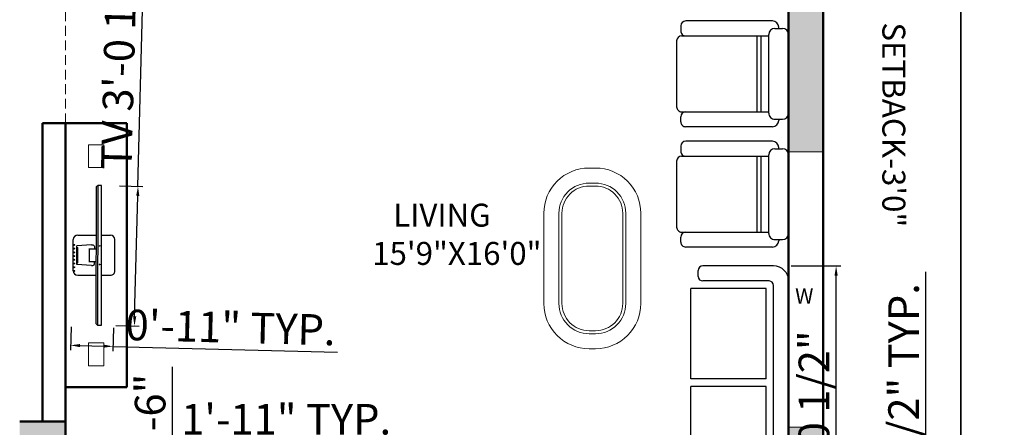
# Model space of a CAD drawing. Units: inches. Extents: x 3354 to 4308, y 1668 to 2317.
# Tile 5 of 11: x 3534 to 3792, y 1960 to 2066. Entities that reach past the tile are written whole.
import ezdxf

# ---------------------------------------------------------------- set-up
doc = ezdxf.new("R2010")
doc.units = ezdxf.units.IN
doc.linetypes.add('DASHED', pattern=[19.05, 12.7, -6.35])
for name, color, linetype, lineweight in [('A-ANNO-DIMS', 2, 'Continuous', 18), ('A-ANNO-TEXT', 7, 'Continuous', 18), ('A-AREA-IDEN', 3, 'Continuous', 18), ('A-FLOR-OVHD', 8, 'DASHED', 18), ('A-FURN', 8, 'Continuous', 18), ('A-GLAZ', 4, 'Continuous', 18), ('A-WALL', 7, 'Continuous', 50), ('A-WALL-PATT', 8, 'Continuous', 13), ('C-PROP', 1, 'Continuous', 35)]:
    doc.layers.add(name, color=color, linetype=linetype, lineweight=lineweight)
for name, color, linetype in [('M40-KOLTUKSUNGERI', 136, 'Continuous'), ('window', 130, 'Continuous'), ('wood', 26, 'Continuous')]:
    doc.layers.add(name, color=color, linetype=linetype)
doc.styles.get("Standard").update_dxf_attribs({"font": 'arial.ttf'})
doc.dimstyles.new('ISO-25', dxfattribs={"dimtxt": 8, "dimasz": 2.5, "dimexe": 1.25, "dimexo": 0.625, "dimtad": 1, "dimdec": 1, "dimlunit": 3, "dimtxsty": 'Standard', "dimcen": 2.5, "dimadec": 0, "dimazin": 0, "dimtfac": 1, "dimtdec": 1, "dimtmove": 0, "dimatfit": 3, "dimfxl": 1, "dimarcsym": 0})

# ---------------------------------------------------------------- blocks, each defined once
blk = doc.blocks.new('TV')
at = {"color": 0}
for p, q in [((3967.27, 1784.85), (3967.05, 1784.65)), ((3967.76, 1763.68), (3967.54, 1763.86))]:
    blk.add_line(p, q, dxfattribs=at)
at = {"layer": 'window'}
for p, q in [((3967.54, 1763.86), (3967.05, 1784.65)), ((3964.41, 1777.23), (3967.22, 1777.3)), ((3968.01, 1777.32), (3969.36, 1777.35)), ((3966.53, 1775.82), (3964.33, 1775.61)), ((3964.34, 1775.34), (3964.45, 1775.34)), ((3964.34, 1775.31), (3964.43, 1775.32)), ((3966.14, 1775.2), (3967.01, 1775.22)), ((3966.14, 1775.18), (3967.27, 1775.2)), ((3966.14, 1775.18), (3966.14, 1775.2)), ((3966.3, 1773.29), (3966.26, 1775.18)), ((3964.39, 1773.06), (3964.48, 1773.06)), ((3964.39, 1773.04), (3964.5, 1773.04)), ((3966.19, 1773.28), (3967.31, 1773.31)), ((3966.19, 1773.26), (3967.05, 1773.28)), ((3966.19, 1773.26), (3966.19, 1773.28)), ((3966.61, 1772.66), (3964.4, 1772.77)), ((3964.55, 1771.15), (3967.36, 1771.22)), ((3968.15, 1771.24), (3969.5, 1771.27))]:
    blk.add_line(p, q, dxfattribs=at)
for points in [[(3968.33, 1763.69), (3967.83, 1784.86), (3967.27, 1784.85), (3967.76, 1763.68), (3968.33, 1763.69)], [(3963.86, 1771.81), (3963.75, 1776.54)], [(3970.16, 1771.96), (3970.05, 1776.69)], [(3964.4, 1772.77), (3964.33, 1775.61)], [(3964.48, 1773.06), (3964.43, 1775.32)], [(3964.5, 1773.04), (3964.45, 1775.34)]]:
    blk.add_lwpolyline(points, dxfattribs=at)
for points in [[(3966.53, 1775.82, -0.263666), (3966.93, 1775.69), (3967, 1775.57), (3967.01, 1775.22)], [(3966.61, 1772.66, 0.263666), (3967, 1772.81), (3967.06, 1772.93), (3967.05, 1773.28)]]:
    blk.add_lwpolyline(points, format="xyb", dxfattribs=at)
for centre, radius in [((3963.91, 1775.73), 0.0679), ((3963.93, 1775.17), 0.0679), ((3963.94, 1774.6), 0.0679), ((3967.77, 1775.68), 0.0451), ((3963.95, 1774.04), 0.0679), ((3963.97, 1773.48), 0.0679), ((3963.98, 1772.92), 0.0679), ((3963.99, 1772.35), 0.0679), ((3964.01, 1771.79), 0.0679), ((3967.83, 1772.86), 0.0451)]:
    blk.add_circle(centre, radius, dxfattribs=at)
for centre, start, end in [((3964.42, 1776.56), 91.3414, 181.3414), ((3969.38, 1776.67), 1.3414, 91.3414), ((3964.53, 1771.83), 181.3414, 271.3414), ((3969.49, 1771.94), 271.3414, 1.3414)]:
    blk.add_arc(centre, 0.676, start, end, dxfattribs=at)
blk = doc.blocks.new('sofa 1')
at = {"layer": 'M40-KOLTUKSUNGERI'}
for p, q in [((72.87, 57.09), (54.36, 57.09)), ((53.18, 54.33), (53.18, 55.91)), ((71.69, 53.15), (54.36, 53.15)), ((72.87, -20.47), (72.87, 51.97)), ((76.8, -21.65), (76.8, 53.15)), ((51.21, 27.56), (51.21, 51.18)), ((70.9, 51.18), (51.21, 51.18)), ((70.9, 27.56), (70.9, 51.18)), ((70.9, 27.56), (51.21, 27.56)), ((51.21, 1.97), (51.21, 25.59)), ((70.9, 25.59), (51.21, 25.59)), ((70.9, 1.97), (70.9, 25.59)), ((0, -19.69), (0, 0)), ((0, -19.69), (0, 0)), ((23.62, 0), (0, 0)), ((23.62, -19.69), (23.62, 0)), ((25.59, -19.69), (25.59, 0)), ((49.21, 0), (25.59, 0)), ((49.21, -19.69), (49.21, 0)), ((70.9, 1.97), (51.21, 1.97)), ((70.9, 0), (51.21, 0)), ((51.21, -19.69), (51.21, 0)), ((70.9, -19.69), (70.9, 0)), ((-3.15, -1.97), (-4.72, -1.97)), ((-5.91, -21.65), (-5.91, -3.15)), ((-1.97, -20.47), (-1.97, -3.15)), ((23.62, -19.69), (0, -19.69)), ((49.21, -19.69), (25.59, -19.69)), ((70.9, -19.69), (51.21, -19.69)), ((71.69, -21.65), (-0.79, -21.65)), ((72.87, -25.59), (-1.97, -25.59))]:
    blk.add_line(p, q, dxfattribs=at)
for centre, radius, start, end in [((54.36, 55.91), 1.18, 90, 180), ((72.87, 53.15), 3.94, 0, 90), ((54.36, 54.33), 1.18, 180, 270), ((71.69, 51.97), 1.18, 0, 90), ((-4.72, -3.15), 1.18, 90, 180), ((-3.15, -3.15), 1.18, 0, 90), ((-0.79, -20.47), 1.18, 180, 270), ((71.69, -20.47), 1.18, 270, 0), ((-1.97, -21.65), 3.94, 180, 270), ((72.87, -21.65), 3.94, 270, 0)]:
    blk.add_arc(centre, radius, start, end, dxfattribs=at)
blk = doc.blocks.new('A$C38B70996')
at = {"layer": 'wood'}
for p, q in [((0.11, 0.9), (0.74, 0.9)), ((0.06, 0.82), (0.05, 0.82)), ((0.06, 0.79), (0.06, 0.85)), ((0.79, 0.79), (0.79, 0.85)), ((0.79, 0.82), (0.8, 0.82)), ((0, 0.77), (0, 0.073)), ((0.74, 0.74), (0.11, 0.74)), ((0.12, 0.04), (0.12, 0.74)), ((0.73, 0.04), (0.73, 0.74)), ((0.85, 0.77), (0.85, 0.073)), ((0.73, 0.68), (0.12, 0.68)), ((0.73, 0.647), (0.12, 0.647)), ((0.04, 0.033), (0.08, 0.033)), ((0.16, 0), (0.69, 0)), ((0.81, 0.033), (0.77, 0.033))]:
    blk.add_line(p, q, dxfattribs=at)
for centre, radius, start, end in [((0.11, 0.85), 0.05, 90, 180), ((0.74, 0.85), 0.05, 0, 90), ((0.05, 0.77), 0.05, 90, 180), ((0.8, 0.77), 0.05, 360, 90), ((0.11, 0.79), 0.05, 180, 270), ((0.74, 0.79), 0.05, 270, 0), ((0.04, 0.073), 0.04, 180, 270), ((0.08, 0.073), 0.04, 270, 0), ((0.16, 0.04), 0.04, 180, 270), ((0.69, 0.04), 0.04, 270, 360), ((0.77, 0.073), 0.04, 180, 270), ((0.81, 0.073), 0.04, 270, 360)]:
    blk.add_arc(centre, radius, start, end, dxfattribs=at)
blk = doc.blocks.new('*D53')
at = {"layer": 'A-ANNO-DIMS', "color": 0, "lineweight": -2, "transparency": 16777216}
for p, q in [((3550.48, 1952.98), (3550.48, 1957.48)), ((3552.98, 1956.23), (3571.19, 1956.23)), ((3573.69, 1952.98), (3573.69, 1957.48)), ((3573.69, 1956.23), (3631.67, 1956.23))]:
    blk.add_line(p, q, dxfattribs=at)
at = {"layer": 'A-ANNO-DIMS', "color": 0, "transparency": 16777216}
for points in [[(3552.98, 1956.64), (3552.98, 1955.81), (3550.48, 1956.23)], [(3571.19, 1956.64), (3571.19, 1955.81), (3573.69, 1956.23)]]:
    blk.add_solid(points, dxfattribs=at)
at = {"layer": 'Defpoints', "color": 0, "transparency": 16777216}
for p in [(3573.69, 1956.23), (3550.48, 1952.36), (3573.69, 1952.36)]:
    blk.add_point(p, dxfattribs=at)
at = {"layer": 'A-ANNO-DIMS', "color": 0, "transparency": 16777216, "insert": (3603.93, 1960.87), "char_height": 8, "attachment_point": 5}
blk.add_mtext('1\'-11" TYP.', dxfattribs=at)
blk = doc.blocks.new('*D66')
at = {"layer": 'A-ANNO-DIMS', "color": 0, "lineweight": -2, "transparency": 16777216}
for p, q in [((3565.2, 2022.8), (3567.45, 2111.51)), ((3560.34, 2022.92), (3566.45, 2022.77)), ((3564.33, 1988.78), (3565.13, 2020.3)), ((3559.42, 1986.4), (3565.52, 1986.25))]:
    blk.add_line(p, q, dxfattribs=at)
at = {"layer": 'A-ANNO-DIMS', "color": 0, "transparency": 16777216}
for points in [[(3564.72, 2020.31), (3565.55, 2020.29), (3565.2, 2022.8)], [(3563.92, 1988.79), (3564.75, 1988.77), (3564.27, 1986.28)]]:
    blk.add_solid(points, dxfattribs=at)
at = {"layer": 'Defpoints', "color": 0, "transparency": 16777216}
for p in [(3559.72, 2022.94), (3565.2, 2022.8), (3558.79, 1986.42)]:
    blk.add_point(p, dxfattribs=at)
at = {"layer": 'A-ANNO-DIMS', "color": 0, "transparency": 16777216, "insert": (3561.6, 2068.53), "char_height": 8, "attachment_point": 5, "rotation": 88.5431}
blk.add_mtext('TV 3\'-0 1/2" TYP.', dxfattribs=at)
blk = doc.blocks.new('*D67')
at = {"layer": 'A-ANNO-DIMS', "color": 0, "lineweight": -2, "transparency": 16777216}
for p, q in [((3547.7, 1986.08), (3547.54, 1979.97)), ((3558.78, 1985.79), (3558.62, 1979.69)), ((3550.07, 1981.16), (3556.15, 1981)), ((3558.65, 1980.94), (3617.36, 1979.45))]:
    blk.add_line(p, q, dxfattribs=at)
at = {"layer": 'A-ANNO-DIMS', "color": 0, "transparency": 16777216}
for points in [[(3550.08, 1981.57), (3550.06, 1980.74), (3547.57, 1981.22)], [(3556.16, 1981.42), (3556.14, 1980.59), (3558.65, 1980.94)]]:
    blk.add_solid(points, dxfattribs=at)
at = {"layer": 'Defpoints', "color": 0, "transparency": 16777216}
for p in [(3547.71, 1986.7), (3558.79, 1986.42), (3558.65, 1980.94)]:
    blk.add_point(p, dxfattribs=at)
at = {"layer": 'A-ANNO-DIMS', "color": 0, "transparency": 16777216, "insert": (3589.38, 1984.87), "char_height": 8, "attachment_point": 5, "rotation": 358.5431}
blk.add_mtext('0\'-11" TYP.', dxfattribs=at)
blk = doc.blocks.new('*D70')
at = {"layer": 'A-ANNO-DIMS', "color": 0, "lineweight": -2, "transparency": 16777216}
for p, q in [((3771.12, 1859.52), (3771.12, 2000.47)), ((3761.34, 1859.52), (3772.37, 1859.52)), ((3771.12, 1792.61), (3771.12, 1857.02)), ((3761.34, 1790.11), (3772.37, 1790.11))]:
    blk.add_line(p, q, dxfattribs=at)
at = {"layer": 'A-ANNO-DIMS', "color": 0, "transparency": 16777216}
for points in [[(3770.71, 1857.02), (3771.54, 1857.02), (3771.12, 1859.52)], [(3770.71, 1792.61), (3771.54, 1792.61), (3771.12, 1790.11)]]:
    blk.add_solid(points, dxfattribs=at)
at = {"layer": 'Defpoints', "color": 0, "transparency": 16777216}
for p in [(3760.71, 1859.52), (3771.12, 1859.52), (3760.71, 1790.11)]:
    blk.add_point(p, dxfattribs=at)
at = {"layer": 'A-ANNO-DIMS', "color": 0, "transparency": 16777216, "insert": (3766.36, 1931.24), "char_height": 8, "attachment_point": 5, "rotation": 90}
blk.add_mtext('MOTORBIKE 5\'-9 1/2" TYP.', dxfattribs=at)
blk = doc.blocks.new('*D74')
at = {"layer": 'A-ANNO-DIMS', "color": 0, "lineweight": -2, "transparency": 16777216}
for p, q in [((3574.18, 1883.3), (3574.18, 1975.62)), ((3581.65, 1883.3), (3572.93, 1883.3)), ((3574.18, 1831.8), (3574.18, 1880.8)), ((3581.65, 1829.3), (3572.93, 1829.3))]:
    blk.add_line(p, q, dxfattribs=at)
at = {"layer": 'A-ANNO-DIMS', "color": 0, "transparency": 16777216}
for points in [[(3573.76, 1880.8), (3574.59, 1880.8), (3574.18, 1883.3)], [(3573.76, 1831.8), (3574.59, 1831.8), (3574.18, 1829.3)]]:
    blk.add_solid(points, dxfattribs=at)
at = {"layer": 'Defpoints', "color": 0, "transparency": 16777216}
for p in [(3574.18, 1883.3), (3582.28, 1883.3), (3582.28, 1829.3)]:
    blk.add_point(p, dxfattribs=at)
at = {"layer": 'A-ANNO-DIMS', "color": 0, "transparency": 16777216, "insert": (3569.41, 1930.71), "char_height": 8, "attachment_point": 5, "rotation": 90}
blk.add_mtext('MAIN DOOR 4\'-6"', dxfattribs=at)
blk = doc.blocks.new('*D87')
at = {"layer": 'A-ANNO-DIMS', "color": 0, "lineweight": -2, "transparency": 16777216}
for p, q in [((3735.9, 2001.97), (3748.93, 2001.97)), ((3747.68, 1921.8), (3747.68, 1999.47)), ((3735.9, 1919.3), (3748.93, 1919.3))]:
    blk.add_line(p, q, dxfattribs=at)
at = {"layer": 'A-ANNO-DIMS', "color": 0, "transparency": 16777216}
for points in [[(3747.27, 1999.47), (3748.1, 1999.47), (3747.68, 2001.97)], [(3747.27, 1921.8), (3748.1, 1921.8), (3747.68, 1919.3)]]:
    blk.add_solid(points, dxfattribs=at)
at = {"layer": 'Defpoints', "color": 0, "transparency": 16777216}
for p in [(3735.28, 2001.97), (3747.68, 2001.97), (3735.28, 1919.3)]:
    blk.add_point(p, dxfattribs=at)
at = {"layer": 'A-ANNO-DIMS', "color": 0, "transparency": 16777216, "insert": (3742.92, 1960.64), "char_height": 8, "attachment_point": 5, "rotation": 90}
blk.add_mtext('6\'-10 1/2"', dxfattribs=at)
blk = doc.blocks.new('*D88')
at = {"layer": 'A-ANNO-DIMS', "color": 0, "lineweight": -2, "transparency": 16777216}
for p, q in [((3405.28, 2080.67), (3405.28, 2074.65)), ((3441.28, 2080.67), (3441.28, 2074.65)), ((3407.78, 2075.9), (3438.78, 2075.9)), ((3441.28, 2075.9), (3543.5, 2075.9))]:
    blk.add_line(p, q, dxfattribs=at)
at = {"layer": 'A-ANNO-DIMS', "color": 0, "transparency": 16777216}
for points in [[(3407.78, 2076.31), (3407.78, 2075.48), (3405.28, 2075.9)], [(3438.78, 2076.31), (3438.78, 2075.48), (3441.28, 2075.9)]]:
    blk.add_solid(points, dxfattribs=at)
at = {"layer": 'Defpoints', "color": 0, "transparency": 16777216}
for p in [(3405.28, 2081.3), (3441.28, 2081.3), (3441.28, 2075.9)]:
    blk.add_point(p, dxfattribs=at)
at = {"layer": 'A-ANNO-DIMS', "color": 0, "transparency": 16777216, "insert": (3493.64, 2080.66), "char_height": 8, "attachment_point": 5}
blk.add_mtext('RANGE OVEN 3\'-0"', dxfattribs=at)

msp = doc.modelspace()

# ---------------------------------------------------------------- hatches: boundary and pattern name
at = {"layer": 'A-WALL-PATT', "transparency": 33554687}
h = msp.add_hatch(color=256, dxfattribs=at)
h.dxf.hatch_style = 1
h.paths.add_polyline_path([(3546.28, 1829.3), (3552.28, 1829.3), (3552.28, 1838.3), (3546.28, 1838.3), (3546.28, 1910.3), (3582.28, 1910.3), (3582.28, 1919.3), (3546.28, 1919.3), (3546.28, 1961.3), (3534.28, 1961.3), (3534.28, 1955.3), (3537.28, 1955.3), (3537.28, 1808.3), (3516.28, 1808.3), (3516.28, 1799.3), (3546.28, 1799.3)])
h.paths.add_polyline_path([(3672.28, 1919.3), (3656.51, 1919.3), (3630.28, 1919.3), (3630.28, 1910.3), (3642.28, 1910.3), (3642.28, 1838.3), (3630.28, 1838.3), (3630.28, 1835.3), (3630.28, 1829.3), (3642.28, 1829.3), (3642.28, 1799.3), (3651.28, 1799.3), (3651.28, 1910.3), (3672.28, 1910.3)])
h.paths.add_polyline_path([(3744.28, 1959.8), (3735.28, 1959.8), (3735.28, 1923.23), (3735.28, 1919.3), (3714.28, 1919.3), (3714.28, 1910.3), (3744.28, 1910.3)])
h.paths.add_polyline_path([(3744.28, 2072.3), (3735.28, 2072.3), (3735.28, 2031.8), (3744.28, 2031.8)])
h.paths.add_polyline_path([(3744.28, 2150.3), (3735.28, 2150.3), (3735.28, 2108.3), (3744.28, 2108.3)])
h.paths.add_polyline_path([(3744.28, 2258.3), (3705.28, 2258.3), (3705.28, 2249.3), (3735.28, 2249.3), (3735.28, 2210.3), (3744.28, 2210.3)])
h.paths.add_polyline_path([(3633.28, 2258.3), (3583.78, 2258.3), (3583.78, 2249.3), (3588.24, 2249.3), (3597.28, 2249.3), (3597.28, 2165.3), (3594.28, 2165.3), (3594.28, 2159.3), (3597.28, 2159.3), (3597.28, 2117.3), (3594.28, 2117.3), (3594.28, 2111.3), (3603.28, 2111.3), (3603.28, 2249.3), (3633.28, 2249.3)])
h.paths.add_polyline_path([(3559.78, 2258.3), (3492.28, 2258.3), (3492.28, 2249.3), (3537.28, 2249.3), (3537.28, 2117.3), (3534.28, 2117.3), (3534.28, 2111.3), (3564.28, 2111.3), (3564.28, 2117.3), (3546.28, 2117.3), (3546.28, 2159.3), (3564.28, 2159.3), (3564.28, 2165.3), (3546.28, 2165.3), (3546.28, 2249.3), (3559.78, 2249.3)])
h.paths.add_polyline_path([(3450.28, 2258.3), (3396.28, 2258.3), (3396.28, 1799.3), (3474.28, 1799.3), (3474.28, 1808.3), (3405.28, 1808.3), (3405.28, 1955.3), (3498.28, 1955.3), (3498.28, 1961.3), (3405.28, 1961.3), (3405.28, 2111.3), (3498.28, 2111.3), (3498.28, 2117.3), (3405.28, 2117.3), (3405.28, 2249.3), (3450.28, 2249.3)])
h.paths.add_polyline_path([(3582.28, 1838.3), (3576.28, 1838.3), (3576.28, 1829.3), (3582.28, 1829.3)], flags=17)

# ---------------------------------------------------------------- linework, layer by layer
at = {"layer": 'A-FLOR-OVHD', "ltscale": 0.2}
msp.add_line((3546.28, 2039.3), (3546.28, 2111.3), dxfattribs=at)
at = {"layer": 'A-FURN'}
for points in [[(3556.28, 2027.67), (3552.28, 2027.67), (3552.28, 2033.67), (3556.28, 2033.67)], [(3556.28, 1981.88), (3552.28, 1981.88), (3552.28, 1975.88), (3556.28, 1975.88)]]:
    msp.add_lwpolyline(points, close=True, dxfattribs=at)
for points in [[(3696.63, 2015.76), (3696.63, 1992.14, -0.414214), (3684.82, 1980.33), (3683.1, 1980.33, -0.414214), (3671.29, 1992.14), (3671.29, 2015.76, -0.414214), (3683.1, 2027.57), (3684.82, 2027.57, -0.414214)], [(3692.7, 2015.76), (3692.7, 1992.14, -0.414214), (3684.82, 1984.26), (3683.1, 1984.26, -0.414214), (3675.23, 1992.14), (3675.23, 2015.76, -0.414214), (3683.1, 2023.63), (3684.82, 2023.63, -0.414214)], [(3691.91, 2015.76), (3691.91, 1992.14, -0.414214), (3684.82, 1985.05), (3683.1, 1985.05, -0.414214), (3676.02, 1992.14), (3676.02, 2015.76, -0.414214), (3683.1, 2022.85), (3684.82, 2022.85, -0.414214)]]:
    msp.add_lwpolyline(points, format="xyb", close=True, dxfattribs=at)
at = {"layer": 'A-GLAZ'}
for p, q in [((3735.28, 2031.8), (3744.28, 2031.8)), ((3735.28, 1959.8), (3744.28, 1959.8))]:
    msp.add_line(p, q, dxfattribs=at)
at = {"layer": 'A-WALL'}
for p, q in [((3735.28, 1919.3), (3735.28, 2072.3)), ((3744.28, 1890.3), (3744.28, 2072.3)), ((3540.28, 2039.3), (3540.28, 1961.3)), ((3546.28, 2039.3), (3540.28, 2039.3)), ((3546.28, 2039.3), (3546.28, 1919.3)), ((3546.28, 2039.3), (3562.28, 2039.3)), ((3562.28, 2039.3), (3562.28, 1970.3)), ((3562.28, 1970.3), (3546.28, 1970.3)), ((3546.28, 1961.3), (3534.28, 1961.3))]:
    msp.add_line(p, q, dxfattribs=at)
at = {"layer": 'C-PROP'}
msp.add_lwpolyline([(3738.28, 1754.3), (3780.28, 1754.3), (3780.28, 2294.3), (3396.28, 2294.3), (3396.28, 1754.3), (3576.28, 1754.3)], dxfattribs=at)

# ---------------------------------------------------------------- block references
at = {"layer": 'A-FURN'}
for name, p, xscale, yscale, zscale, rotation in [('A$C38B70996', (3706, 2066.02), 32.53084308163255, 32.53084308163255, 32.53084308163255, 270), ('A$C38B70996', (3706, 2034.57), 32.53084308163255, 32.53084308163255, 32.53084308163255, 270), ('TV', (-3362.83, -879.97), 1.724488909621177, 1.724488909621177, 1.724488909621177, 358.5430845181614)]:
    msp.add_blockref(name, p, dxfattribs=dict(at, xscale=xscale, yscale=yscale, zscale=zscale, rotation=rotation))
msp.add_blockref('sofa 1', (3658.47, 1944.89), dxfattribs=at)

# ---------------------------------------------------------------- texts
at = {"layer": 'A-ANNO-TEXT', "insert": (3765.77, 2065.64), "char_height": 6, "attachment_point": 1, "rotation": 270}
msp.add_mtext_dynamic_manual_height_columns('{SETBACK-3\'0"}', width=74.5832, gutter_width=12.5, heights=[0], dxfattribs=at)
at = {"layer": 'A-ANNO-TEXT', "insert": (3736.97, 1996.14), "char_height": 4, "attachment_point": 1}
msp.add_mtext_dynamic_manual_height_columns('\\pxt6;{W}', width=32.7844, gutter_width=12.5, heights=[0], dxfattribs=at)
at = {"layer": 'A-AREA-IDEN', "insert": (3626.41, 2018.25), "char_height": 6, "attachment_point": 1}
msp.add_mtext_dynamic_manual_height_columns('   LIVING\\P15\'9"X16\'0"', width=74.5832, gutter_width=12.5, heights=[0], dxfattribs=at)

# ---------------------------------------------------------------- dimensions: what is measured, and where the dimension line sits
at = {"layer": 'A-ANNO-DIMS'}
for base, p1, p2, angle, text, picture, middle in [((3565.2, 2022.8), (3558.79, 1986.42), (3559.72, 2022.94), 88.5431, 'TV <> TYP.', '*D66', (3561.6, 2068.53)), ((3771.12, 1859.52), (3760.71, 1790.11), (3760.71, 1859.52), 90, 'MOTORBIKE <> TYP.', '*D70', (3766.36, 1931.24)), ((3558.65, 1980.94), (3547.71, 1986.7), (3558.79, 1986.42), 358.5431, '<> TYP.', '*D67', (3589.38, 1984.87)), ((3574.18, 1883.3), (3582.28, 1829.3), (3582.28, 1883.3), 90, 'MAIN DOOR <>', '*D74', (3569.41, 1930.71))]:
    dim = msp.add_linear_dim(base=base, p1=p1, p2=p2, angle=angle, text=text, dimstyle='ISO-25', override={"dimdec": 1, "dimrnd": 0, "dimzin": 1, "dimlunit": 4, "dimfrac": 2}, dxfattribs=at)
    dim.commit()
    dim.dimension.update_dxf_attribs({"geometry": picture, "text_midpoint": middle})
for base, p1, p2, text, picture, middle in [((3441.28, 2075.9), (3405.28, 2081.3), (3441.28, 2081.3), 'RANGE OVEN <>', '*D88', (3493.64, 2080.66)), ((3573.69, 1956.23), (3550.48, 1952.36), (3573.69, 1952.36), '<> TYP.', '*D53', (3603.93, 1960.87))]:
    dim = msp.add_linear_dim(base=base, p1=p1, p2=p2, text=text, dimstyle='ISO-25', override={"dimdec": 1, "dimrnd": 0, "dimzin": 1, "dimlunit": 4, "dimfrac": 2}, dxfattribs=at)
    dim.commit()
    dim.dimension.update_dxf_attribs({"geometry": picture, "text_midpoint": middle})
dim = msp.add_linear_dim(base=(3747.68, 2001.97), p1=(3735.28, 1919.3), p2=(3735.28, 2001.97), angle=90, dimstyle='ISO-25', override={"dimdec": 1, "dimrnd": 0, "dimzin": 1, "dimlunit": 4, "dimfrac": 2}, dxfattribs=at)
dim.commit()
dim.dimension.update_dxf_attribs({"geometry": '*D87', "text_midpoint": (3742.92, 1960.64)})

doc.saveas('drawing.dxf')
